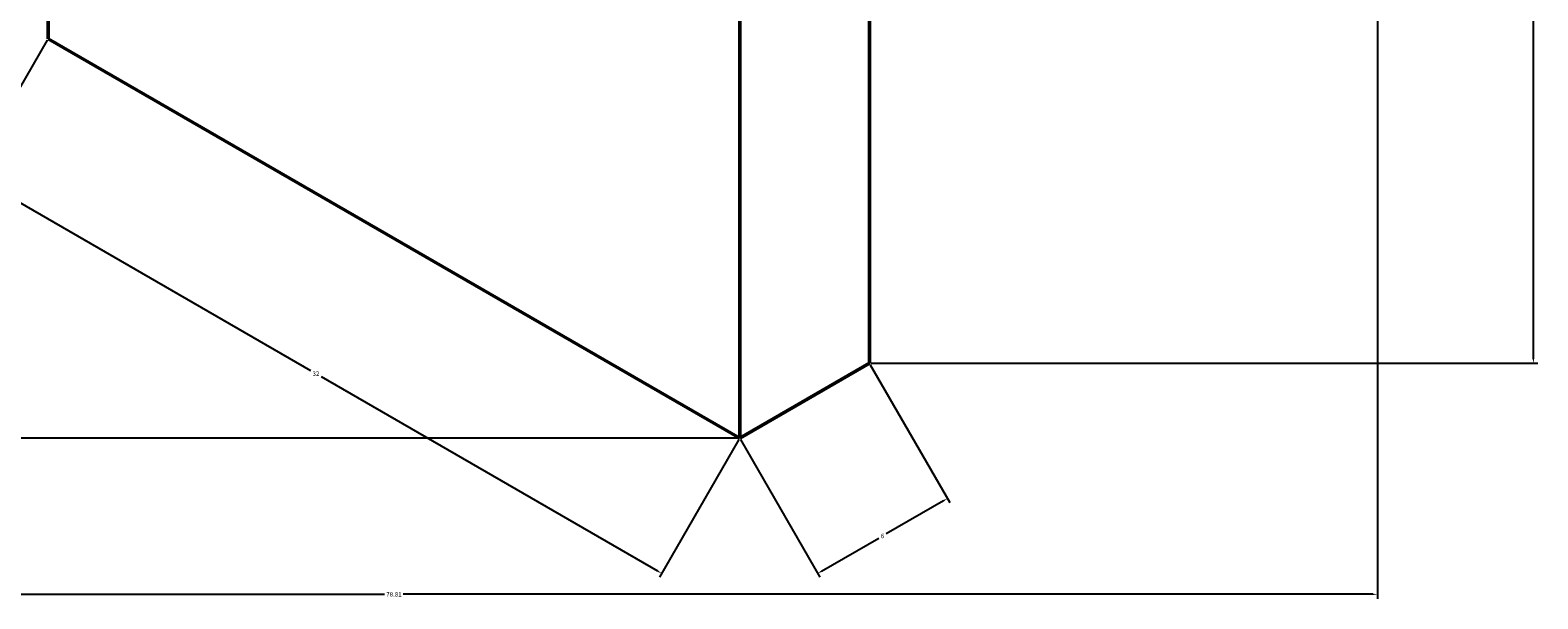
# Model space of a CAD drawing. Units: inches. Extents: x -23 to 69, y -27 to 96.
# Tile 2 of 10: x 8 to 69, y -27 to -5. Entities that reach past the tile are written whole.
import ezdxf

# ---------------------------------------------------------------- set-up
doc = ezdxf.new("R2010")
doc.units = ezdxf.units.IN
doc.header["$MEASUREMENT"] = 0
doc.layers.add('M-DIMS', color=2, linetype='Continuous', lineweight=18)
doc.layers.add('M-OUTL', color=7, linetype='Continuous', lineweight=50)
doc.styles.get("Standard").update_dxf_attribs({"font": 'arial.ttf'})
doc.dimstyles.get("Standard").update_dxf_attribs({"dimtxt": 0.18, "dimasz": 0.18, "dimexe": 0.18, "dimexo": 0.0625, "dimgap": 0.09, "dimtad": 0, "dimtih": 1, "dimtoh": 1, "dimdec": 4, "dimzin": 0, "dimdsep": 46, "dimtxsty": 'Standard', "dimcen": 0.09, "dimadec": 0, "dimazin": 0, "dimtfac": 1, "dimtdec": 4, "dimtofl": 0, "dimtmove": 0, "dimatfit": 3, "dimfxl": 1, "dimtolj": 1, "dimtzin": 0, "dimarcsym": 0})

# ---------------------------------------------------------------- blocks, each defined once
blk = doc.blocks.new('*D4')
at = {"layer": 'Defpoints', "color": 0, "transparency": 16777216}
for p in [(41.819, 16.119), (68.421, 16.119), (41.819, -17.881)]:
    blk.add_point(p, dxfattribs=at)
at = {"layer": 'M-DIMS', "color": 0, "lineweight": -2, "transparency": 16777216}
for p, q in [((41.881, 16.119), (68.601, 16.119)), ((68.421, 15.939), (68.421, -0.699)), ((68.421, -17.701), (68.421, -1.063)), ((41.881, -17.881), (68.601, -17.881))]:
    blk.add_line(p, q, dxfattribs=at)
at = {"layer": 'M-DIMS', "color": 0, "transparency": 16777216}
for points in [[(68.391, 15.939), (68.451, 15.939), (68.421, 16.119)], [(68.391, -17.701), (68.451, -17.701), (68.421, -17.881)]]:
    blk.add_solid(points, dxfattribs=at)
at = {"layer": 'M-DIMS', "color": 0, "transparency": 16777216, "insert": (68.421, -0.881), "char_height": 0.18, "attachment_point": 5}
blk.add_mtext('\\A1;34', dxfattribs=at)
blk = doc.blocks.new('*D5')
at = {"layer": 'Defpoints', "color": 0, "transparency": 16777216}
for p in [(41.819, -17.881), (36.623, -20.881), (39.748, -26.294)]:
    blk.add_point(p, dxfattribs=at)
at = {"layer": 'M-DIMS', "color": 0, "lineweight": -2, "transparency": 16777216}
for p, q in [((41.85, -17.935), (45.034, -23.45)), ((36.654, -20.935), (39.838, -26.45)), ((44.788, -23.384), (42.495, -24.708)), ((39.904, -26.204), (42.196, -24.88))]:
    blk.add_line(p, q, dxfattribs=at)
at = {"layer": 'M-DIMS', "color": 0, "transparency": 16777216}
for points in [[(44.773, -23.358), (44.803, -23.41), (44.944, -23.294)], [(39.889, -26.178), (39.919, -26.23), (39.748, -26.294)]]:
    blk.add_solid(points, dxfattribs=at)
at = {"layer": 'M-DIMS', "color": 0, "transparency": 16777216, "insert": (42.346, -24.794), "char_height": 0.18, "attachment_point": 5}
blk.add_mtext('\\A1;6', dxfattribs=at)
blk = doc.blocks.new('*D6')
at = {"layer": 'Defpoints', "color": 0, "transparency": 16777216}
for p in [(8.91, -4.881), (5.785, -10.294), (36.623, -20.881)]:
    blk.add_point(p, dxfattribs=at)
at = {"layer": 'M-DIMS', "color": 0, "lineweight": -2, "transparency": 16777216}
for p, q in [((8.879, -4.935), (5.695, -10.45)), ((5.941, -10.384), (19.423, -18.168)), ((33.342, -26.204), (19.859, -18.42)), ((36.592, -20.935), (33.408, -26.45))]:
    blk.add_line(p, q, dxfattribs=at)
at = {"layer": 'M-DIMS', "color": 0, "transparency": 16777216}
for points in [[(5.956, -10.358), (5.926, -10.41), (5.785, -10.294)], [(33.357, -26.178), (33.327, -26.23), (33.498, -26.294)]]:
    blk.add_solid(points, dxfattribs=at)
at = {"layer": 'M-DIMS', "color": 0, "transparency": 16777216, "insert": (19.641, -18.294), "char_height": 0.18, "attachment_point": 5}
blk.add_mtext('\\A1;32', dxfattribs=at)
blk = doc.blocks.new('*D13')
at = {"layer": 'Defpoints', "color": 0, "transparency": 16777216}
for p in [(15.838, 89.119), (-22.888, -20.881), (36.623, -20.881)]:
    blk.add_point(p, dxfattribs=at)
at = {"layer": 'M-DIMS', "color": 0, "lineweight": -2, "transparency": 16777216}
for p, q in [((15.776, 89.119), (-23.068, 89.119)), ((-22.888, 88.939), (-22.888, 34.301)), ((-22.888, -20.701), (-22.888, 33.937)), ((36.56, -20.881), (-23.068, -20.881))]:
    blk.add_line(p, q, dxfattribs=at)
at = {"layer": 'M-DIMS', "color": 0, "transparency": 16777216}
for points in [[(-22.918, 88.939), (-22.858, 88.939), (-22.888, 89.119)], [(-22.918, -20.701), (-22.858, -20.701), (-22.888, -20.881)]]:
    blk.add_solid(points, dxfattribs=at)
at = {"layer": 'M-DIMS', "color": 0, "transparency": 16777216, "insert": (-22.888, 34.119), "char_height": 0.18, "attachment_point": 5}
blk.add_mtext('\\A1;110', dxfattribs=at)
blk = doc.blocks.new('*D17')
at = {"layer": 'Defpoints', "color": 0, "transparency": 16777216}
for p in [(62.171, 27.869), (-16.638, 20.369), (62.171, -27.131)]:
    blk.add_point(p, dxfattribs=at)
at = {"layer": 'M-DIMS', "color": 0, "lineweight": -2, "transparency": 16777216}
for p, q in [((62.171, 27.806), (62.171, -27.311)), ((-16.638, 20.306), (-16.638, -27.311)), ((-16.458, -27.131), (22.391, -27.131)), ((61.991, -27.131), (23.142, -27.131))]:
    blk.add_line(p, q, dxfattribs=at)
at = {"layer": 'M-DIMS', "color": 0, "transparency": 16777216}
for points in [[(-16.458, -27.101), (-16.458, -27.161), (-16.638, -27.131)], [(61.991, -27.101), (61.991, -27.161), (62.171, -27.131)]]:
    blk.add_solid(points, dxfattribs=at)
at = {"layer": 'M-DIMS', "color": 0, "transparency": 16777216, "insert": (22.766, -27.131), "char_height": 0.18, "attachment_point": 5}
blk.add_mtext('\\A1;78.81', dxfattribs=at)

msp = doc.modelspace()

# ---------------------------------------------------------------- linework, layer by layer
at = {"layer": 'M-OUTL'}
for p, q in [((41.819, -17.8814), (41.819, 16.1186)), ((36.6228, 13.1186), (36.6228, -20.8814)), ((8.91, -4.8814), (8.91, 5.6186)), ((36.6228, -20.8814), (8.91, -4.8814)), ((36.6228, -20.8814), (41.819, -17.8814))]:
    msp.add_line(p, q, dxfattribs=at)

# ---------------------------------------------------------------- dimensions: what is measured, and where the dimension line sits
at = {"layer": 'M-DIMS'}
for base, p1, p2, angle, picture, middle in [((-22.8877, -20.8814), (15.8382, 89.1186), (36.6228, -20.8814), 90, '*D13', (-22.8877, 34.1186)), ((68.4206, 16.1186), (41.819, -17.8814), (41.819, 16.1186), 90, '*D4', (68.4206, -0.8814)), ((5.785, -10.294), (36.6228, -20.8814), (8.91, -4.8814), 150, '*D6', (19.6414, -18.294)), ((39.7478, -26.294), (41.819, -17.8814), (36.6228, -20.8814), 210, '*D5', (42.3459, -24.794))]:
    dim = msp.add_linear_dim(base=base, p1=p1, p2=p2, angle=angle, dimstyle='Standard', override={"dimdec": 0, "dimlfac": 1, "dimrnd": 0, "dimzin": 0, "dimdsep": 46, "dimlunit": 2}, dxfattribs=at)
    dim.commit()
    dim.dimension.update_dxf_attribs({"geometry": picture, "text_midpoint": middle})
dim = msp.add_linear_dim(base=(62.1706, -27.1314), p1=(-16.6377, 20.3686), p2=(62.1706, 27.8686), dimstyle='Standard', override={"dimdec": 2, "dimlfac": 1, "dimrnd": 0, "dimzin": 0, "dimdsep": 46, "dimlunit": 2}, dxfattribs=at)
dim.commit()
dim.dimension.update_dxf_attribs({"geometry": '*D17', "text_midpoint": (22.7664, -27.1314)})

doc.saveas('drawing.dxf')
